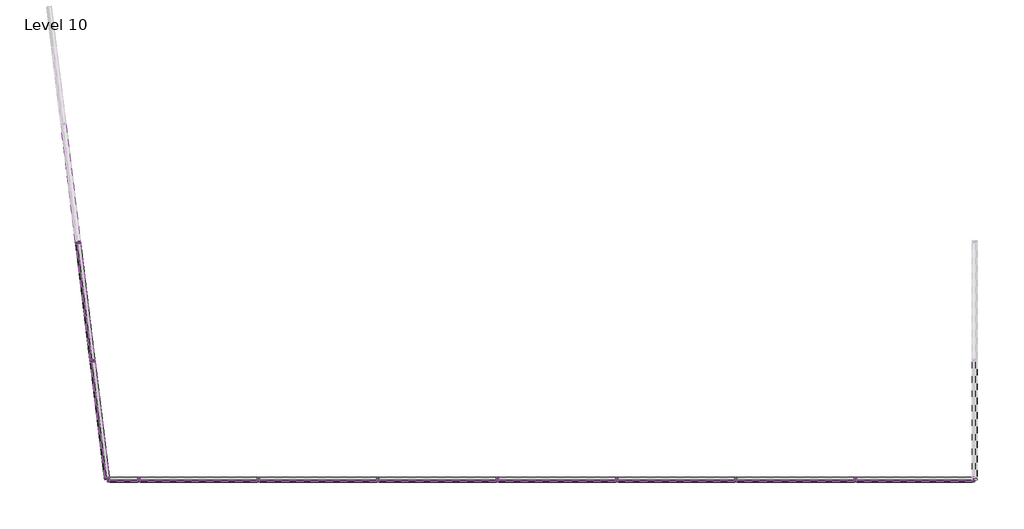
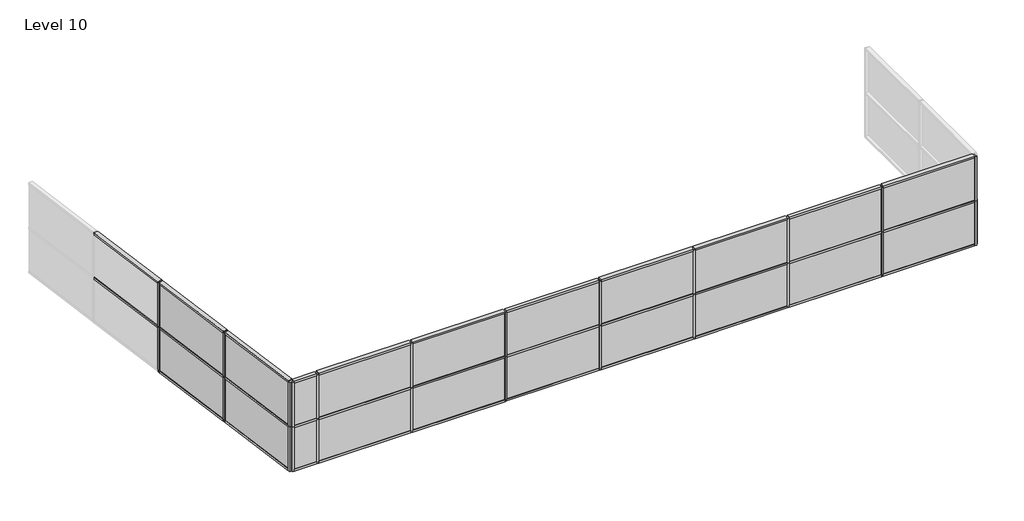
# One storey, part 1 of 2: 70 members, 24 plates.
"""IFC4 building model written with IfcOpenShell, lengths in millimetres."""

from ifc_helpers import new_model, si_unit, origin, place, context, project, spatial, transform, mapped, element, save
from components import member_71c27fd2, member_19d0a4ec, member_8cef0660, member_db480205, member_82905deb, member_4491d118, member_695b83e4, member_0c11e56c, system_panel_glazed_37f15d2e, system_panel_glazed_3620f98e, system_panel_glazed_e46d4b42, system_panel_glazed_2a6c68b7, system_panel_glazed_07b088f8, system_panel_glazed_9d0e0944

model = new_model("IFC4")

# Units and contexts
model_context = context("Model", 3, world=origin())
ifc_project = project(units=[si_unit("LENGTHUNIT", "METRE", prefix="MILLI")], contexts=[model_context])

# Site, building, storey
site = spatial("IfcSite", under=ifc_project)
building = spatial("IfcBuilding", under=site)
storey = spatial("IfcBuildingStorey", under=building, Name="Level 10", Elevation=27432.0)

# Members
placement = place(None, origin())
member_shape = member_71c27fd2(model_context)
element("IfcMember", 1, ObjectType="Rectangular Mullion : 2.5\" x 5\" rectangular", at=placement, inside=storey, context=model_context, shape_type="MappedRepresentation", body=[
    mapped(member_shape, transform((-8620.3262186, -3985.3690403, 27432.0), x_axis=(0.0, 0.0, -1.0), y_axis=(-0.9925461516413222, -0.12186934340514607, 0.0), z_axis=(-0.12186934340514607, 0.9925461516413222, 0.0))),
])
element("IfcMember", 2, ObjectType="Rectangular Mullion : 2.5\" x 5\" rectangular", at=placement, inside=storey, context=model_context, shape_type="MappedRepresentation", body=[
    mapped(member_shape, transform((10886.265636, -6979.1363705, 27432.0), x_axis=(0.0, 0.0, -1.0), y_axis=(0.0, -1.0, 0.0), z_axis=(-1.0, 0.0, 0.0))),
])
element("IfcMember", 3, ObjectType="Rectangular Mullion : 2.5\" x 5\" rectangular", at=placement, inside=storey, context=model_context, shape_type="MappedRepresentation", body=[
    mapped(member_shape, transform((13902.5156363, -6915.6363705, 27432.0), x_axis=(0.0, 0.0, -1.0), y_axis=(1.0, 0.0, 0.0), z_axis=(0.0, -1.0, 0.0))),
])
member_2_shape = member_19d0a4ec(model_context)
element("IfcMember", 4, ObjectType="Rectangular Mullion : 2.5\" x 5\" rectangular", at=placement, inside=storey, context=model_context, shape_type="MappedRepresentation", body=[
    mapped(member_2_shape, transform((-8260.4765148, -6916.1096898, 28956.0), x_axis=(0.0, 0.0, 1.0), y_axis=(-0.9925461516413222, -0.12186934340514598, 0.0), z_axis=(0.12186934340514596, -0.9925461516413221, 0.0))),
])
element("IfcMember", 5, ObjectType="Rectangular Mullion : 2.5\" x 5\" rectangular", at=placement, inside=storey, context=model_context, shape_type="MappedRepresentation", body=[
    mapped(member_2_shape, transform((-8260.4765148, -6916.1096898, 30480.0), x_axis=(0.0, 0.0, 1.0), y_axis=(-0.9925461516413222, -0.12186934340514585, 0.0), z_axis=(0.12186934340514584, -0.9925461516413221, 0.0))),
])
element("IfcMember", 6, ObjectType="Rectangular Mullion : 2.5\" x 5\" rectangular", at=placement, inside=storey, context=model_context, shape_type="MappedRepresentation", body=[
    mapped(member_2_shape, transform((-8260.4765148, -6916.1096898, 28956.0), x_axis=(0.0, 0.0, 1.0), y_axis=(-0.9925461516413222, -0.12186934340514587, 0.0), z_axis=(0.12186934340514587, -0.9925461516413222, 0.0))),
])
element("IfcMember", 7, ObjectType="Rectangular Mullion : 2.5\" x 5\" rectangular", at=placement, inside=storey, context=model_context, shape_type="MappedRepresentation", body=[
    mapped(member_2_shape, transform((-8260.4765148, -6916.1096898, 30480.0), x_axis=(0.0, 0.0, 1.0), y_axis=(-0.9925461516413223, -0.12186934340514574, 0.0), z_axis=(0.12186934340514574, -0.9925461516413223, 0.0))),
])
element("IfcMember", 8, ObjectType="Rectangular Mullion : 2.5\" x 5\" rectangular", at=placement, inside=storey, context=model_context, shape_type="MappedRepresentation", body=[
    mapped(member_2_shape, transform((13839.0156363, -6979.1363705, 28956.0), x_axis=(0.0, 0.0, 1.0), y_axis=(0.0, -1.0, 0.0), z_axis=(1.0, 0.0, 0.0))),
])
element("IfcMember", 9, ObjectType="Rectangular Mullion : 2.5\" x 5\" rectangular", at=placement, inside=storey, context=model_context, shape_type="MappedRepresentation", body=[
    mapped(member_2_shape, transform((13839.0156363, -6979.1363705, 30480.0), x_axis=(0.0, 0.0, 1.0), y_axis=(0.0, -1.0, 0.0), z_axis=(1.0, 0.0, 0.0))),
])
member_3_shape = member_8cef0660(model_context)
element("IfcMember", 10, ObjectType="Rectangular Mullion : 2.5\" x 5\" rectangular", at=placement, inside=storey, context=model_context, shape_type="MappedRepresentation", body=[
    mapped(member_3_shape, transform((-8628.0649219, -3922.3423596, 28956.0), x_axis=(0.0, 0.0, 1.0), y_axis=(-0.9925461516413222, -0.12186934340514595, 0.0), z_axis=(0.12186934340514595, -0.9925461516413222, 0.0))),
])
element("IfcMember", 11, ObjectType="Rectangular Mullion : 2.5\" x 5\" rectangular", at=placement, inside=storey, context=model_context, shape_type="MappedRepresentation", body=[
    mapped(member_3_shape, transform((-8999.5226806, -897.0616894, 28956.0), x_axis=(0.0, 0.0, 1.0), y_axis=(-0.9925461516413222, -0.12186934340514602, 0.0), z_axis=(0.12186934340514602, -0.9925461516413222, 0.0))),
])
element("IfcMember", 12, ObjectType="Rectangular Mullion : 2.5\" x 5\" rectangular", at=placement, inside=storey, context=model_context, shape_type="MappedRepresentation", body=[
    mapped(member_3_shape, transform((-8628.0649219, -3922.3423596, 30480.0), x_axis=(0.0, 0.0, 1.0), y_axis=(-0.9925461516413222, -0.12186934340514595, 0.0), z_axis=(0.12186934340514595, -0.9925461516413222, 0.0))),
])
element("IfcMember", 13, ObjectType="Rectangular Mullion : 2.5\" x 5\" rectangular", at=placement, inside=storey, context=model_context, shape_type="MappedRepresentation", body=[
    mapped(member_3_shape, transform((-8999.5226806, -897.0616894, 30480.0), x_axis=(0.0, 0.0, 1.0), y_axis=(-0.9925461516413222, -0.12186934340514566, 0.0), z_axis=(0.12186934340514566, -0.9925461516413222, 0.0))),
])
element("IfcMember", 14, ObjectType="Rectangular Mullion : 2.5\" x 5\" rectangular", at=placement, inside=storey, context=model_context, shape_type="MappedRepresentation", body=[
    mapped(member_3_shape, transform((-8628.0649219, -3922.3423596, 28956.0), x_axis=(0.0, 0.0, 1.0), y_axis=(-0.9925461516413223, -0.12186934340514574, 0.0), z_axis=(0.12186934340514574, -0.9925461516413223, 0.0))),
])
element("IfcMember", 15, ObjectType="Rectangular Mullion : 2.5\" x 5\" rectangular", at=placement, inside=storey, context=model_context, shape_type="MappedRepresentation", body=[
    mapped(member_3_shape, transform((-8999.5226806, -897.0616894, 28956.0), x_axis=(0.0, 0.0, 1.0), y_axis=(-0.9925461516413222, -0.12186934340514592, 0.0), z_axis=(0.12186934340514592, -0.9925461516413222, 0.0))),
])
element("IfcMember", 16, ObjectType="Rectangular Mullion : 2.5\" x 5\" rectangular", at=placement, inside=storey, context=model_context, shape_type="MappedRepresentation", body=[
    mapped(member_3_shape, transform((-8628.0649219, -3922.3423596, 30480.0), x_axis=(0.0, 0.0, 1.0), y_axis=(-0.9925461516413222, -0.12186934340514606, 0.0), z_axis=(0.12186934340514606, -0.9925461516413222, 0.0))),
])
element("IfcMember", 17, ObjectType="Rectangular Mullion : 2.5\" x 5\" rectangular", at=placement, inside=storey, context=model_context, shape_type="MappedRepresentation", body=[
    mapped(member_3_shape, transform((-8999.5226806, -897.0616894, 30480.0), x_axis=(0.0, 0.0, 1.0), y_axis=(-0.9925461516413222, -0.12186934340514595, 0.0), z_axis=(0.12186934340514595, -0.9925461516413222, 0.0))),
])
element("IfcMember", 18, ObjectType="Rectangular Mullion : 2.5\" x 5\" rectangular", at=placement, inside=storey, context=model_context, shape_type="MappedRepresentation", body=[
    mapped(member_3_shape, transform((10822.765636, -6979.1363705, 28956.0), x_axis=(0.0, 0.0, 1.0), y_axis=(0.0, -1.0, 0.0), z_axis=(1.0, 0.0, 0.0))),
])
element("IfcMember", 19, ObjectType="Rectangular Mullion : 2.5\" x 5\" rectangular", at=placement, inside=storey, context=model_context, shape_type="MappedRepresentation", body=[
    mapped(member_3_shape, transform((7774.765636, -6979.1363705, 28956.0), x_axis=(0.0, 0.0, 1.0), y_axis=(0.0, -1.0, 0.0), z_axis=(1.0, 0.0, 0.0))),
])
element("IfcMember", 20, ObjectType="Rectangular Mullion : 2.5\" x 5\" rectangular", at=placement, inside=storey, context=model_context, shape_type="MappedRepresentation", body=[
    mapped(member_3_shape, transform((4726.765636, -6979.1363705, 28956.0), x_axis=(0.0, 0.0, 1.0), y_axis=(0.0, -1.0, 0.0), z_axis=(1.0, 0.0, 0.0))),
])
element("IfcMember", 21, ObjectType="Rectangular Mullion : 2.5\" x 5\" rectangular", at=placement, inside=storey, context=model_context, shape_type="MappedRepresentation", body=[
    mapped(member_3_shape, transform((1678.765636, -6979.1363705, 28956.0), x_axis=(0.0, 0.0, 1.0), y_axis=(0.0, -1.0, 0.0), z_axis=(1.0, 0.0, 0.0))),
])
element("IfcMember", 22, ObjectType="Rectangular Mullion : 2.5\" x 5\" rectangular", at=placement, inside=storey, context=model_context, shape_type="MappedRepresentation", body=[
    mapped(member_3_shape, transform((-1369.234364, -6979.1363705, 28956.0), x_axis=(0.0, 0.0, 1.0), y_axis=(0.0, -1.0, 0.0), z_axis=(1.0, 0.0, 0.0))),
])
element("IfcMember", 23, ObjectType="Rectangular Mullion : 2.5\" x 5\" rectangular", at=placement, inside=storey, context=model_context, shape_type="MappedRepresentation", body=[
    mapped(member_3_shape, transform((-4417.234364, -6979.1363705, 28956.0), x_axis=(0.0, 0.0, 1.0), y_axis=(0.0, -1.0, 0.0), z_axis=(1.0, 0.0, 0.0))),
])
element("IfcMember", 24, ObjectType="Rectangular Mullion : 2.5\" x 5\" rectangular", at=placement, inside=storey, context=model_context, shape_type="MappedRepresentation", body=[
    mapped(member_3_shape, transform((10822.765636, -6979.1363705, 30480.0), x_axis=(0.0, 0.0, 1.0), y_axis=(0.0, -1.0, 0.0), z_axis=(1.0, 0.0, 0.0))),
])
element("IfcMember", 25, ObjectType="Rectangular Mullion : 2.5\" x 5\" rectangular", at=placement, inside=storey, context=model_context, shape_type="MappedRepresentation", body=[
    mapped(member_3_shape, transform((7774.765636, -6979.1363705, 30480.0), x_axis=(0.0, 0.0, 1.0), y_axis=(0.0, -1.0, 0.0), z_axis=(1.0, 0.0, 0.0))),
])
element("IfcMember", 26, ObjectType="Rectangular Mullion : 2.5\" x 5\" rectangular", at=placement, inside=storey, context=model_context, shape_type="MappedRepresentation", body=[
    mapped(member_3_shape, transform((4726.765636, -6979.1363705, 30480.0), x_axis=(0.0, 0.0, 1.0), y_axis=(0.0, -1.0, 0.0), z_axis=(1.0, 0.0, 0.0))),
])
element("IfcMember", 27, ObjectType="Rectangular Mullion : 2.5\" x 5\" rectangular", at=placement, inside=storey, context=model_context, shape_type="MappedRepresentation", body=[
    mapped(member_3_shape, transform((1678.765636, -6979.1363705, 30480.0), x_axis=(0.0, 0.0, 1.0), y_axis=(0.0, -1.0, 0.0), z_axis=(1.0, 0.0, 0.0))),
])
element("IfcMember", 28, ObjectType="Rectangular Mullion : 2.5\" x 5\" rectangular", at=placement, inside=storey, context=model_context, shape_type="MappedRepresentation", body=[
    mapped(member_3_shape, transform((-1369.234364, -6979.1363705, 30480.0), x_axis=(0.0, 0.0, 1.0), y_axis=(0.0, -1.0, 0.0), z_axis=(1.0, 0.0, 0.0))),
])
element("IfcMember", 29, ObjectType="Rectangular Mullion : 2.5\" x 5\" rectangular", at=placement, inside=storey, context=model_context, shape_type="MappedRepresentation", body=[
    mapped(member_3_shape, transform((-4417.234364, -6979.1363705, 30480.0), x_axis=(0.0, 0.0, 1.0), y_axis=(0.0, -1.0, 0.0), z_axis=(1.0, 0.0, 0.0))),
])
member_4_shape = member_db480205(model_context)
element("IfcMember", 30, ObjectType="Rectangular Mullion : 2.5\" x 5\" rectangular", at=placement, inside=storey, context=model_context, shape_type="MappedRepresentation", body=[
    mapped(member_4_shape, transform((-8991.7839773, -960.0883701, 27432.0), x_axis=(0.0, 0.0, -1.0), y_axis=(-0.9925461516413222, -0.12186934340514607, 0.0), z_axis=(-0.12186934340514607, 0.9925461516413222, 0.0))),
])
element("IfcMember", 31, ObjectType="Rectangular Mullion : 2.5\" x 5\" rectangular", at=placement, inside=storey, context=model_context, shape_type="MappedRepresentation", body=[
    mapped(member_4_shape, transform((7838.265636, -6979.1363705, 27432.0), x_axis=(0.0, 0.0, -1.0), y_axis=(0.0, -1.0, 0.0), z_axis=(-1.0, 0.0, 0.0))),
])
element("IfcMember", 32, ObjectType="Rectangular Mullion : 2.5\" x 5\" rectangular", at=placement, inside=storey, context=model_context, shape_type="MappedRepresentation", body=[
    mapped(member_4_shape, transform((4790.265636, -6979.1363705, 27432.0), x_axis=(0.0, 0.0, -1.0), y_axis=(0.0, -1.0, 0.0), z_axis=(-1.0, 0.0, 0.0))),
])
element("IfcMember", 33, ObjectType="Rectangular Mullion : 2.5\" x 5\" rectangular", at=placement, inside=storey, context=model_context, shape_type="MappedRepresentation", body=[
    mapped(member_4_shape, transform((1742.265636, -6979.1363705, 27432.0), x_axis=(0.0, 0.0, -1.0), y_axis=(0.0, -1.0, 0.0), z_axis=(-1.0, 0.0, 0.0))),
])
element("IfcMember", 34, ObjectType="Rectangular Mullion : 2.5\" x 5\" rectangular", at=placement, inside=storey, context=model_context, shape_type="MappedRepresentation", body=[
    mapped(member_4_shape, transform((-1305.734364, -6979.1363705, 27432.0), x_axis=(0.0, 0.0, -1.0), y_axis=(0.0, -1.0, 0.0), z_axis=(-1.0, 0.0, 0.0))),
])
element("IfcMember", 35, ObjectType="Rectangular Mullion : 2.5\" x 5\" rectangular", at=placement, inside=storey, context=model_context, shape_type="MappedRepresentation", body=[
    mapped(member_4_shape, transform((-4353.734364, -6979.1363705, 27432.0), x_axis=(0.0, 0.0, -1.0), y_axis=(0.0, -1.0, 0.0), z_axis=(-1.0, 0.0, 0.0))),
])
element("IfcMember", 36, ObjectType="Rectangular Mullion : 2.5\" x 5\" rectangular", at=placement, inside=storey, context=model_context, shape_type="MappedRepresentation", body=[
    mapped(member_4_shape, transform((-7401.734364, -6979.1363705, 27432.0), x_axis=(0.0, 0.0, -1.0), y_axis=(0.0, -1.0, 0.0), z_axis=(-1.0, 0.0, 0.0))),
])
member_5_shape = member_82905deb(model_context)
element("IfcMember", 37, ObjectType="Rectangular Mullion : 2.5\" x 5\" rectangular", at=placement, inside=storey, context=model_context, shape_type="MappedRepresentation", body=[
    mapped(member_5_shape, transform((-8624.1955702, -3953.8557, 28956.0), x_axis=(-0.1218693434051459, 0.9925461516413222, 0.0), y_axis=(-0.9925461516413222, -0.1218693434051459, 0.0), z_axis=(0.0, 0.0, 1.0))),
])
element("IfcMember", 38, ObjectType="Rectangular Mullion : 2.5\" x 5\" rectangular", at=placement, inside=storey, context=model_context, shape_type="MappedRepresentation", body=[
    mapped(member_5_shape, transform((-8995.6533289, -928.5750297, 28956.0), x_axis=(-0.1218693434051459, 0.9925461516413222, 0.0), y_axis=(-0.9925461516413222, -0.1218693434051459, 0.0), z_axis=(0.0, 0.0, 1.0))),
])
element("IfcMember", 39, ObjectType="Rectangular Mullion : 2.5\" x 5\" rectangular", at=placement, inside=storey, context=model_context, shape_type="MappedRepresentation", body=[
    mapped(member_5_shape, transform((10854.515636, -6979.1363705, 28956.0), x_axis=(-1.0, 0.0, 0.0), y_axis=(0.0, -1.0, 0.0), z_axis=(0.0, 0.0, 1.0))),
])
element("IfcMember", 40, ObjectType="Rectangular Mullion : 2.5\" x 5\" rectangular", at=placement, inside=storey, context=model_context, shape_type="MappedRepresentation", body=[
    mapped(member_5_shape, transform((7806.515636, -6979.1363705, 28956.0), x_axis=(-1.0, 0.0, 0.0), y_axis=(0.0, -1.0, 0.0), z_axis=(0.0, 0.0, 1.0))),
])
element("IfcMember", 41, ObjectType="Rectangular Mullion : 2.5\" x 5\" rectangular", at=placement, inside=storey, context=model_context, shape_type="MappedRepresentation", body=[
    mapped(member_5_shape, transform((4758.515636, -6979.1363705, 28956.0), x_axis=(-1.0, 0.0, 0.0), y_axis=(0.0, -1.0, 0.0), z_axis=(0.0, 0.0, 1.0))),
])
element("IfcMember", 42, ObjectType="Rectangular Mullion : 2.5\" x 5\" rectangular", at=placement, inside=storey, context=model_context, shape_type="MappedRepresentation", body=[
    mapped(member_5_shape, transform((1710.515636, -6979.1363705, 28956.0), x_axis=(-1.0, 0.0, 0.0), y_axis=(0.0, -1.0, 0.0), z_axis=(0.0, 0.0, 1.0))),
])
element("IfcMember", 43, ObjectType="Rectangular Mullion : 2.5\" x 5\" rectangular", at=placement, inside=storey, context=model_context, shape_type="MappedRepresentation", body=[
    mapped(member_5_shape, transform((-1337.484364, -6979.1363705, 28956.0), x_axis=(-1.0, 0.0, 0.0), y_axis=(0.0, -1.0, 0.0), z_axis=(0.0, 0.0, 1.0))),
])
element("IfcMember", 44, ObjectType="Rectangular Mullion : 2.5\" x 5\" rectangular", at=placement, inside=storey, context=model_context, shape_type="MappedRepresentation", body=[
    mapped(member_5_shape, transform((-4385.484364, -6979.1363705, 28956.0), x_axis=(-1.0, 0.0, 0.0), y_axis=(0.0, -1.0, 0.0), z_axis=(0.0, 0.0, 1.0))),
])
element("IfcMember", 45, ObjectType="Rectangular Mullion : 2.5\" x 5\" rectangular", at=placement, inside=storey, context=model_context, shape_type="MappedRepresentation", body=[
    mapped(member_5_shape, transform((-7433.484364, -6979.1363705, 28956.0), x_axis=(-1.0, 0.0, 0.0), y_axis=(0.0, -1.0, 0.0), z_axis=(0.0, 0.0, 1.0))),
])
element("IfcMember", 46, ObjectType="Rectangular Mullion : 2.5\" x 5\" rectangular", at=placement, inside=storey, context=model_context, shape_type="MappedRepresentation", body=[
    mapped(member_5_shape, transform((-8624.1955702, -3953.8557, 28956.0), x_axis=(-0.1218693434051459, 0.9925461516413222, 0.0), y_axis=(-0.9925461516413222, -0.1218693434051459, 0.0), z_axis=(0.0, 0.0, 1.0))),
])
element("IfcMember", 47, ObjectType="Rectangular Mullion : 2.5\" x 5\" rectangular", at=placement, inside=storey, context=model_context, shape_type="MappedRepresentation", body=[
    mapped(member_5_shape, transform((-8624.1955702, -3953.8557, 30480.0), x_axis=(-0.1218693434051459, 0.9925461516413222, 0.0), y_axis=(-0.9925461516413222, -0.1218693434051459, 0.0), z_axis=(0.0, 0.0, 1.0))),
])
element("IfcMember", 48, ObjectType="Rectangular Mullion : 2.5\" x 5\" rectangular", at=placement, inside=storey, context=model_context, shape_type="MappedRepresentation", body=[
    mapped(member_5_shape, transform((-8995.6533289, -928.5750297, 28956.0), x_axis=(-0.1218693434051459, 0.9925461516413222, 0.0), y_axis=(-0.9925461516413222, -0.1218693434051459, 0.0), z_axis=(0.0, 0.0, 1.0))),
])
element("IfcMember", 49, ObjectType="Rectangular Mullion : 2.5\" x 5\" rectangular", at=placement, inside=storey, context=model_context, shape_type="MappedRepresentation", body=[
    mapped(member_5_shape, transform((-8995.6533289, -928.5750297, 30480.0), x_axis=(-0.1218693434051459, 0.9925461516413222, 0.0), y_axis=(-0.9925461516413222, -0.1218693434051459, 0.0), z_axis=(0.0, 0.0, 1.0))),
])
element("IfcMember", 50, ObjectType="Rectangular Mullion : 2.5\" x 5\" rectangular", at=placement, inside=storey, context=model_context, shape_type="MappedRepresentation", body=[
    mapped(member_5_shape, transform((-8624.1955702, -3953.8557, 30480.0), x_axis=(-0.1218693434051459, 0.9925461516413222, 0.0), y_axis=(-0.9925461516413222, -0.1218693434051459, 0.0), z_axis=(0.0, 0.0, 1.0))),
])
element("IfcMember", 51, ObjectType="Rectangular Mullion : 2.5\" x 5\" rectangular", at=placement, inside=storey, context=model_context, shape_type="MappedRepresentation", body=[
    mapped(member_5_shape, transform((-8995.6533289, -928.5750297, 30480.0), x_axis=(-0.1218693434051459, 0.9925461516413222, 0.0), y_axis=(-0.9925461516413222, -0.1218693434051459, 0.0), z_axis=(0.0, 0.0, 1.0))),
])
element("IfcMember", 52, ObjectType="Rectangular Mullion : 2.5\" x 5\" rectangular", at=placement, inside=storey, context=model_context, shape_type="MappedRepresentation", body=[
    mapped(member_5_shape, transform((10854.515636, -6979.1363705, 30480.0), x_axis=(-1.0, 0.0, 0.0), y_axis=(0.0, -1.0, 0.0), z_axis=(0.0, 0.0, 1.0))),
])
element("IfcMember", 53, ObjectType="Rectangular Mullion : 2.5\" x 5\" rectangular", at=placement, inside=storey, context=model_context, shape_type="MappedRepresentation", body=[
    mapped(member_5_shape, transform((7806.515636, -6979.1363705, 30480.0), x_axis=(-1.0, 0.0, 0.0), y_axis=(0.0, -1.0, 0.0), z_axis=(0.0, 0.0, 1.0))),
])
element("IfcMember", 54, ObjectType="Rectangular Mullion : 2.5\" x 5\" rectangular", at=placement, inside=storey, context=model_context, shape_type="MappedRepresentation", body=[
    mapped(member_5_shape, transform((4758.515636, -6979.1363705, 30480.0), x_axis=(-1.0, 0.0, 0.0), y_axis=(0.0, -1.0, 0.0), z_axis=(0.0, 0.0, 1.0))),
])
element("IfcMember", 55, ObjectType="Rectangular Mullion : 2.5\" x 5\" rectangular", at=placement, inside=storey, context=model_context, shape_type="MappedRepresentation", body=[
    mapped(member_5_shape, transform((1710.515636, -6979.1363705, 30480.0), x_axis=(-1.0, 0.0, 0.0), y_axis=(0.0, -1.0, 0.0), z_axis=(0.0, 0.0, 1.0))),
])
element("IfcMember", 56, ObjectType="Rectangular Mullion : 2.5\" x 5\" rectangular", at=placement, inside=storey, context=model_context, shape_type="MappedRepresentation", body=[
    mapped(member_5_shape, transform((-1337.484364, -6979.1363705, 30480.0), x_axis=(-1.0, 0.0, 0.0), y_axis=(0.0, -1.0, 0.0), z_axis=(0.0, 0.0, 1.0))),
])
element("IfcMember", 57, ObjectType="Rectangular Mullion : 2.5\" x 5\" rectangular", at=placement, inside=storey, context=model_context, shape_type="MappedRepresentation", body=[
    mapped(member_5_shape, transform((-4385.484364, -6979.1363705, 30480.0), x_axis=(-1.0, 0.0, 0.0), y_axis=(0.0, -1.0, 0.0), z_axis=(0.0, 0.0, 1.0))),
])
element("IfcMember", 58, ObjectType="Rectangular Mullion : 2.5\" x 5\" rectangular", at=placement, inside=storey, context=model_context, shape_type="MappedRepresentation", body=[
    mapped(member_5_shape, transform((-7433.484364, -6979.1363705, 30480.0), x_axis=(-1.0, 0.0, 0.0), y_axis=(0.0, -1.0, 0.0), z_axis=(0.0, 0.0, 1.0))),
])
member_6_shape = member_4491d118(model_context)
element("IfcMember", 59, ObjectType="Rectangular Mullion : 2.5\" x 5\" rectangular", at=placement, inside=storey, context=model_context, shape_type="MappedRepresentation", body=[
    mapped(member_6_shape, transform((-8252.7378115, -6979.1363705, 27432.0), x_axis=(0.1218693434051459, -0.9925461516413222, 0.0), y_axis=(-0.9925461516413222, -0.1218693434051459, 0.0), z_axis=(0.0, 0.0, -1.0))),
])
element("IfcMember", 60, ObjectType="Rectangular Mullion : 2.5\" x 5\" rectangular", at=placement, inside=storey, context=model_context, shape_type="MappedRepresentation", body=[
    mapped(member_6_shape, transform((13902.5156363, -6979.1363705, 27432.0), x_axis=(1.0, 0.0, 0.0), y_axis=(0.0, -1.0, 0.0), z_axis=(0.0, 0.0, -1.0))),
])
element("IfcMember", 61, ObjectType="Rectangular Mullion : 2.5\" x 5\" rectangular", at=placement, inside=storey, context=model_context, shape_type="MappedRepresentation", body=[
    mapped(member_6_shape, transform((-8252.7378115, -6979.1363705, 27432.0), x_axis=(0.1218693434051459, -0.9925461516413222, 0.0), y_axis=(-0.9925461516413222, -0.1218693434051459, 0.0), z_axis=(0.0, 0.0, -1.0))),
])
element("IfcMember", 62, ObjectType="Rectangular Mullion : 2.5\" x 5\" rectangular", at=placement, inside=storey, context=model_context, shape_type="MappedRepresentation", body=[
    mapped(member_6_shape, transform((-8252.7378115, -6979.1363705, 28956.0), x_axis=(0.1218693434051459, -0.9925461516413222, 0.0), y_axis=(-0.9925461516413222, -0.1218693434051459, 0.0), z_axis=(0.0, 0.0, -1.0))),
])
element("IfcMember", 63, ObjectType="Rectangular Mullion : 2.5\" x 5\" rectangular", at=placement, inside=storey, context=model_context, shape_type="MappedRepresentation", body=[
    mapped(member_6_shape, transform((-8252.7378115, -6979.1363705, 28956.0), x_axis=(0.1218693434051459, -0.9925461516413222, 0.0), y_axis=(-0.9925461516413222, -0.1218693434051459, 0.0), z_axis=(0.0, 0.0, -1.0))),
])
element("IfcMember", 64, ObjectType="Rectangular Mullion : 2.5\" x 5\" rectangular", at=placement, inside=storey, context=model_context, shape_type="MappedRepresentation", body=[
    mapped(member_6_shape, transform((13902.5156363, -6979.1363705, 28956.0), x_axis=(1.0, 0.0, 0.0), y_axis=(0.0, -1.0, 0.0), z_axis=(0.0, 0.0, -1.0))),
])
element("IfcMember", 65, ObjectType="Rectangular Mullion : 2.5\" x 5\" rectangular", at=placement, inside=storey, context=model_context, shape_type="MappedRepresentation", body=[
    mapped(member_6_shape, transform((-8252.7378115, -6979.1363705, 28956.0), x_axis=(-1.0, 0.0, 0.0), y_axis=(0.0, -1.0, 0.0), z_axis=(0.0, 0.0, 1.0))),
])
element("IfcMember", 66, ObjectType="Rectangular Mullion : 2.5\" x 5\" rectangular", at=placement, inside=storey, context=model_context, shape_type="MappedRepresentation", body=[
    mapped(member_6_shape, transform((13902.5156363, -6979.1363705, 28956.0), x_axis=(0.0, -1.0, 0.0), y_axis=(1.0, 0.0, 0.0), z_axis=(0.0, 0.0, 1.0))),
])
element("IfcMember", 67, ObjectType="Rectangular Mullion : 2.5\" x 5\" rectangular", at=placement, inside=storey, context=model_context, shape_type="MappedRepresentation", body=[
    mapped(member_6_shape, transform((-8252.7378115, -6979.1363705, 30480.0), x_axis=(-1.0, 0.0, 0.0), y_axis=(0.0, -1.0, 0.0), z_axis=(0.0, 0.0, 1.0))),
])
member_7_shape = member_695b83e4(model_context)
element("IfcMember", 68, ObjectType="Rectangular Mullion : 2.5\" x 5\" rectangular", at=placement, inside=storey, context=model_context, shape_type="MappedRepresentation", body=[
    mapped(member_7_shape, transform((-8189.2378115, -6979.1363705, 27432.0), x_axis=(0.0, 0.0, -1.0), y_axis=(0.0, -1.0, 0.0), z_axis=(-1.0, 0.0, 0.0))),
])
member_8_shape = member_0c11e56c(model_context)
element("IfcMember", 69, ObjectType="Rectangular Mullion : 2.5\" x 5\" rectangular", at=placement, inside=storey, context=model_context, shape_type="MappedRepresentation", body=[
    mapped(member_8_shape, transform((-7465.234364, -6979.1363705, 28956.0), x_axis=(0.0, 0.0, 1.0), y_axis=(0.0, -1.0, 0.0), z_axis=(1.0, 0.0, 0.0))),
])
element("IfcMember", 70, ObjectType="Rectangular Mullion : 2.5\" x 5\" rectangular", at=placement, inside=storey, context=model_context, shape_type="MappedRepresentation", body=[
    mapped(member_8_shape, transform((-7465.234364, -6979.1363705, 30480.0), x_axis=(0.0, 0.0, 1.0), y_axis=(0.0, -1.0, 0.0), z_axis=(1.0, 0.0, 0.0))),
])

# Plates
system_panel_glazed_shape = system_panel_glazed_37f15d2e(model_context)
element("IfcPlate", 71, ObjectType="System Panel : Glazed", at=placement, inside=storey, context=model_context, shape_type="MappedRepresentation", body=[
    mapped(system_panel_glazed_shape, transform((-8440.4013667, -5450.739365, 27495.5), x_axis=(-0.1218693434051459, 0.9925461516413222, 0.0), y_axis=(-0.9925461516413222, -0.1218693434051459, 0.0), z_axis=(0.0, 0.0, 1.0))),
])
element("IfcPlate", 72, ObjectType="System Panel : Glazed", at=placement, inside=storey, context=model_context, shape_type="MappedRepresentation", body=[
    mapped(system_panel_glazed_shape, transform((12362.6406361, -6979.1363705, 27495.5), x_axis=(-1.0, 0.0, 0.0), y_axis=(0.0, -1.0, 0.0), z_axis=(0.0, 0.0, 1.0))),
])
system_panel_glazed_2_shape = system_panel_glazed_3620f98e(model_context)
element("IfcPlate", 73, ObjectType="System Panel : Glazed", at=placement, inside=storey, context=model_context, shape_type="MappedRepresentation", body=[
    mapped(system_panel_glazed_2_shape, transform((-8809.9244496, -2441.2153649, 27495.5), x_axis=(-0.1218693434051459, 0.9925461516413222, 0.0), y_axis=(-0.9925461516413222, -0.1218693434051459, 0.0), z_axis=(0.0, 0.0, 1.0))),
])
element("IfcPlate", 74, ObjectType="System Panel : Glazed", at=placement, inside=storey, context=model_context, shape_type="MappedRepresentation", body=[
    mapped(system_panel_glazed_2_shape, transform((9330.515636, -6979.1363705, 27495.5), x_axis=(-1.0, 0.0, 0.0), y_axis=(0.0, -1.0, 0.0), z_axis=(0.0, 0.0, 1.0))),
])
element("IfcPlate", 75, ObjectType="System Panel : Glazed", at=placement, inside=storey, context=model_context, shape_type="MappedRepresentation", body=[
    mapped(system_panel_glazed_2_shape, transform((6282.515636, -6979.1363705, 27495.5), x_axis=(-1.0, 0.0, 0.0), y_axis=(0.0, -1.0, 0.0), z_axis=(0.0, 0.0, 1.0))),
])
element("IfcPlate", 76, ObjectType="System Panel : Glazed", at=placement, inside=storey, context=model_context, shape_type="MappedRepresentation", body=[
    mapped(system_panel_glazed_2_shape, transform((3234.515636, -6979.1363705, 27495.5), x_axis=(-1.0, 0.0, 0.0), y_axis=(0.0, -1.0, 0.0), z_axis=(0.0, 0.0, 1.0))),
])
element("IfcPlate", 77, ObjectType="System Panel : Glazed", at=placement, inside=storey, context=model_context, shape_type="MappedRepresentation", body=[
    mapped(system_panel_glazed_2_shape, transform((186.515636, -6979.1363705, 27495.5), x_axis=(-1.0, 0.0, 0.0), y_axis=(0.0, -1.0, 0.0), z_axis=(0.0, 0.0, 1.0))),
])
element("IfcPlate", 78, ObjectType="System Panel : Glazed", at=placement, inside=storey, context=model_context, shape_type="MappedRepresentation", body=[
    mapped(system_panel_glazed_2_shape, transform((-2861.484364, -6979.1363705, 27495.5), x_axis=(-1.0, 0.0, 0.0), y_axis=(0.0, -1.0, 0.0), z_axis=(0.0, 0.0, 1.0))),
])
element("IfcPlate", 79, ObjectType="System Panel : Glazed", at=placement, inside=storey, context=model_context, shape_type="MappedRepresentation", body=[
    mapped(system_panel_glazed_2_shape, transform((-5909.484364, -6979.1363705, 27495.5), x_axis=(-1.0, 0.0, 0.0), y_axis=(0.0, -1.0, 0.0), z_axis=(0.0, 0.0, 1.0))),
])
system_panel_glazed_3_shape = system_panel_glazed_e46d4b42(model_context)
element("IfcPlate", 80, ObjectType="System Panel : Glazed", at=placement, inside=storey, context=model_context, shape_type="MappedRepresentation", body=[
    mapped(system_panel_glazed_3_shape, transform((-8440.4013667, -5450.739365, 27463.75), x_axis=(-0.1218693434051459, 0.9925461516413222, 0.0), y_axis=(-0.9925461516413222, -0.1218693434051459, 0.0), z_axis=(0.0, 0.0, 1.0))),
])
element("IfcPlate", 81, ObjectType="System Panel : Glazed", at=placement, inside=storey, context=model_context, shape_type="MappedRepresentation", body=[
    mapped(system_panel_glazed_3_shape, transform((-8440.4013667, -5450.739365, 28987.75), x_axis=(-0.1218693434051459, 0.9925461516413222, 0.0), y_axis=(-0.9925461516413222, -0.1218693434051459, 0.0), z_axis=(0.0, 0.0, 1.0))),
])
element("IfcPlate", 82, ObjectType="System Panel : Glazed", at=placement, inside=storey, context=model_context, shape_type="MappedRepresentation", body=[
    mapped(system_panel_glazed_3_shape, transform((-8440.4013667, -5450.739365, 28987.75), x_axis=(-0.1218693434051459, 0.9925461516413222, 0.0), y_axis=(-0.9925461516413222, -0.1218693434051459, 0.0), z_axis=(0.0, 0.0, 1.0))),
])
element("IfcPlate", 83, ObjectType="System Panel : Glazed", at=placement, inside=storey, context=model_context, shape_type="MappedRepresentation", body=[
    mapped(system_panel_glazed_3_shape, transform((12362.6406361, -6979.1363705, 28987.75), x_axis=(-1.0, 0.0, 0.0), y_axis=(0.0, -1.0, 0.0), z_axis=(0.0, 0.0, 1.0))),
])
system_panel_glazed_4_shape = system_panel_glazed_2a6c68b7(model_context)
element("IfcPlate", 84, ObjectType="System Panel : Glazed", at=placement, inside=storey, context=model_context, shape_type="MappedRepresentation", body=[
    mapped(system_panel_glazed_4_shape, transform((-8809.9244496, -2441.2153649, 27463.75), x_axis=(-0.1218693434051459, 0.9925461516413222, 0.0), y_axis=(-0.9925461516413222, -0.1218693434051459, 0.0), z_axis=(0.0, 0.0, 1.0))),
])
element("IfcPlate", 85, ObjectType="System Panel : Glazed", at=placement, inside=storey, context=model_context, shape_type="MappedRepresentation", body=[
    mapped(system_panel_glazed_4_shape, transform((-8809.9244496, -2441.2153649, 28987.75), x_axis=(-0.1218693434051459, 0.9925461516413222, 0.0), y_axis=(-0.9925461516413222, -0.1218693434051459, 0.0), z_axis=(0.0, 0.0, 1.0))),
])
element("IfcPlate", 86, ObjectType="System Panel : Glazed", at=placement, inside=storey, context=model_context, shape_type="MappedRepresentation", body=[
    mapped(system_panel_glazed_4_shape, transform((-8809.9244496, -2441.2153649, 28987.75), x_axis=(-0.1218693434051459, 0.9925461516413222, 0.0), y_axis=(-0.9925461516413222, -0.1218693434051459, 0.0), z_axis=(0.0, 0.0, 1.0))),
])
element("IfcPlate", 87, ObjectType="System Panel : Glazed", at=placement, inside=storey, context=model_context, shape_type="MappedRepresentation", body=[
    mapped(system_panel_glazed_4_shape, transform((9330.515636, -6979.1363705, 28987.75), x_axis=(-1.0, 0.0, 0.0), y_axis=(0.0, -1.0, 0.0), z_axis=(0.0, 0.0, 1.0))),
])
element("IfcPlate", 88, ObjectType="System Panel : Glazed", at=placement, inside=storey, context=model_context, shape_type="MappedRepresentation", body=[
    mapped(system_panel_glazed_4_shape, transform((6282.515636, -6979.1363705, 28987.75), x_axis=(-1.0, 0.0, 0.0), y_axis=(0.0, -1.0, 0.0), z_axis=(0.0, 0.0, 1.0))),
])
element("IfcPlate", 89, ObjectType="System Panel : Glazed", at=placement, inside=storey, context=model_context, shape_type="MappedRepresentation", body=[
    mapped(system_panel_glazed_4_shape, transform((3234.515636, -6979.1363705, 28987.75), x_axis=(-1.0, 0.0, 0.0), y_axis=(0.0, -1.0, 0.0), z_axis=(0.0, 0.0, 1.0))),
])
element("IfcPlate", 90, ObjectType="System Panel : Glazed", at=placement, inside=storey, context=model_context, shape_type="MappedRepresentation", body=[
    mapped(system_panel_glazed_4_shape, transform((186.515636, -6979.1363705, 28987.75), x_axis=(-1.0, 0.0, 0.0), y_axis=(0.0, -1.0, 0.0), z_axis=(0.0, 0.0, 1.0))),
])
element("IfcPlate", 91, ObjectType="System Panel : Glazed", at=placement, inside=storey, context=model_context, shape_type="MappedRepresentation", body=[
    mapped(system_panel_glazed_4_shape, transform((-2861.484364, -6979.1363705, 28987.75), x_axis=(-1.0, 0.0, 0.0), y_axis=(0.0, -1.0, 0.0), z_axis=(0.0, 0.0, 1.0))),
])
element("IfcPlate", 92, ObjectType="System Panel : Glazed", at=placement, inside=storey, context=model_context, shape_type="MappedRepresentation", body=[
    mapped(system_panel_glazed_4_shape, transform((-5909.484364, -6979.1363705, 28987.75), x_axis=(-1.0, 0.0, 0.0), y_axis=(0.0, -1.0, 0.0), z_axis=(0.0, 0.0, 1.0))),
])
system_panel_glazed_5_shape = system_panel_glazed_07b088f8(model_context)
element("IfcPlate", 93, ObjectType="System Panel : Glazed", at=placement, inside=storey, context=model_context, shape_type="MappedRepresentation", body=[
    mapped(system_panel_glazed_5_shape, transform((-7827.2360878, -6979.1363705, 27495.5), x_axis=(-1.0, 0.0, 0.0), y_axis=(0.0, -1.0, 0.0), z_axis=(0.0, 0.0, 1.0))),
])
system_panel_glazed_6_shape = system_panel_glazed_9d0e0944(model_context)
element("IfcPlate", 94, ObjectType="System Panel : Glazed", at=placement, inside=storey, context=model_context, shape_type="MappedRepresentation", body=[
    mapped(system_panel_glazed_6_shape, transform((-7827.2360878, -6979.1363705, 28987.75), x_axis=(-1.0, 0.0, 0.0), y_axis=(0.0, -1.0, 0.0), z_axis=(0.0, 0.0, 1.0))),
])

save(model, "model.ifc")

# Revit data of these elements
# Type "Rectangular Mullion : 2.5\" x 5\" rectangular"
#   built-in parameter 1007304 = 0.416667 (stored number, unit not read)
#   built-in parameter 1007301 = 0.104167 (stored number, unit not read)
#   built-in parameter 1007300 = 0.104167 (stored number, unit not read)
# Type "System Panel : Glazed"
#   Construction Type Id = "GSP4R"
#   Analytic Construction = "1/8 in Pilkington single glazing"
#   Visual Light Transmittance = 0.9
#   Solar Heat Gain Coefficient = 0.86
#   Heat Transfer Coefficient (U) = 1.18115 BTU/(h·ft²·°F)
#   Define Thermal Properties by = 1
# Elements 1, 2, 3, 4, 5, 6, 7, 8, 9, 10, 11, 12, 13, 14, 15, 16, 17, 18, 19, 20, 21, 22, 23, 24, 25, 26, 27, 28, 29, 30, 31, 32, 33, 34, 35, 36, 37, 38, 39, 40, 41, 42, 43, 44, 45, 46, 47, 48, 49, 50, 51, 52, 53, 54, 55, 56, 57, 58, 59, 60, 61, 62, 63, 64, 65, 66, 67, 68, 69, 70 (IfcMember, "Rectangular Mullion : 2.5\" x 5\" rectangular")
#   Phase Created = New Construction
#   Materials on its faces: "Aluminum"
# Elements 71, 72, 73, 74, 75, 76, 77, 78, 79, 80, 81, 82, 83, 84, 85, 86, 87, 88, 89, 90, 91, 92, 93, 94 (IfcPlate, "System Panel : Glazed")
#   Phase Created = New Construction
#   Materials on its faces: "Glass"
# Materials
#   "Aluminum": class "Metal", colour RGB 247 247 247, transparency 0, Description = "Aluminum 6061", Cost = 0
#   "Glass": class "Glass", colour RGB 0 128 192, transparency 0.75, Description = "Soda Lime Glass", Cost = 0
